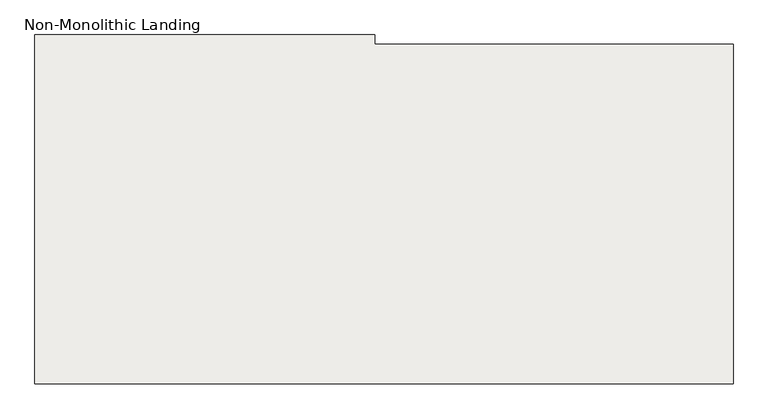
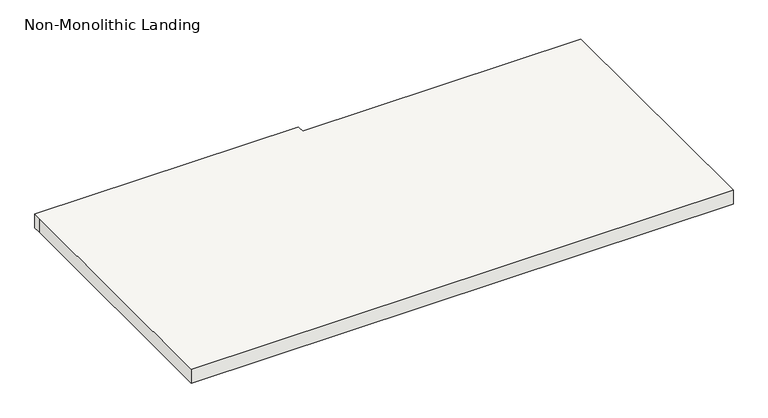
"""IFC4 building model written with IfcOpenShell, lengths in millimetres: slab geometry, Non-Monolithic Landing."""

from ifc_helpers import new_model, si_unit, origin, place, context, project, spatial, faceted_brep, source, transform, mapped, element, save


def non_monolithic_landing_2d37ff17(model_context):
    return source(origin(), model_context, "Body", "Brep", [
        faceted_brep([(-3400.7137331, -6527.0593836, 1504.95), (-3400.7137331, -6552.4593836, 1479.55), (-4315.1137331, -6552.4593836, 1479.55), (-4315.1137331, -6527.0593836, 1504.95), (-4365.9137331, -6527.0593836, 1524.0), (-4365.9137331, -6501.6593836, 1524.0), (-5280.3137331, -6501.6593836, 1524.0), (-5280.3137331, -6527.0593836, 1524.0), (-5280.3137331, -7441.4593836, 1524.0), (-3400.7137331, -7441.4593836, 1524.0), (-3400.7137331, -6527.0593836, 1524.0), (-4315.1137331, -6552.4593836, 1473.2), (-3400.7137331, -6552.4593836, 1473.2), (-3400.7137331, -7441.4593836, 1473.2), (-5280.3137331, -7441.4593836, 1473.2), (-5280.3137331, -6527.0593836, 1473.2), (-5280.3137331, -6501.6593836, 1473.2), (-4365.9137331, -6501.6593836, 1473.2), (-4365.9137331, -6527.0593836, 1473.2), (-4315.1137331, -6527.0593836, 1473.2)], [[[0, 1, 2, 3]], [[4, 5, 6, 7, 8, 9, 10]], [[11, 12, 13, 14, 15, 16, 17, 18, 19]], [[12, 11, 2, 1]], [[11, 19, 3, 2]], [[4, 10, 0, 3, 19, 18]], [[5, 4, 18, 17]], [[6, 5, 17, 16]], [[7, 6, 16, 15]], [[8, 7, 15, 14]], [[9, 8, 14, 13]], [[10, 9, 13, 12, 1, 0]]]),
    ])


if __name__ == "__main__":
    model = new_model("IFC4")
    model_context = context("Model", 3, world=origin())
    ifc_project = project(units=[si_unit("LENGTHUNIT", "METRE", prefix="MILLI")], contexts=[model_context])
    site = spatial("IfcSite", under=ifc_project)
    building = spatial("IfcBuilding", under=site)
    placement = place(None, origin())
    non_monolithic_landing_shape = non_monolithic_landing_2d37ff17(model_context)
    element("IfcSlab", 1, ObjectType="Non-Monolithic Landing", at=placement, inside=building, context=model_context, shape_type="MappedRepresentation", body=[
        mapped(non_monolithic_landing_shape, transform((0.0, 0.0, 0.0), x_axis=(1.0, 0.0, 0.0), y_axis=(0.0, 1.0, 0.0), z_axis=(0.0, 0.0, 1.0))),
    ])
    save(model, "model.ifc")
